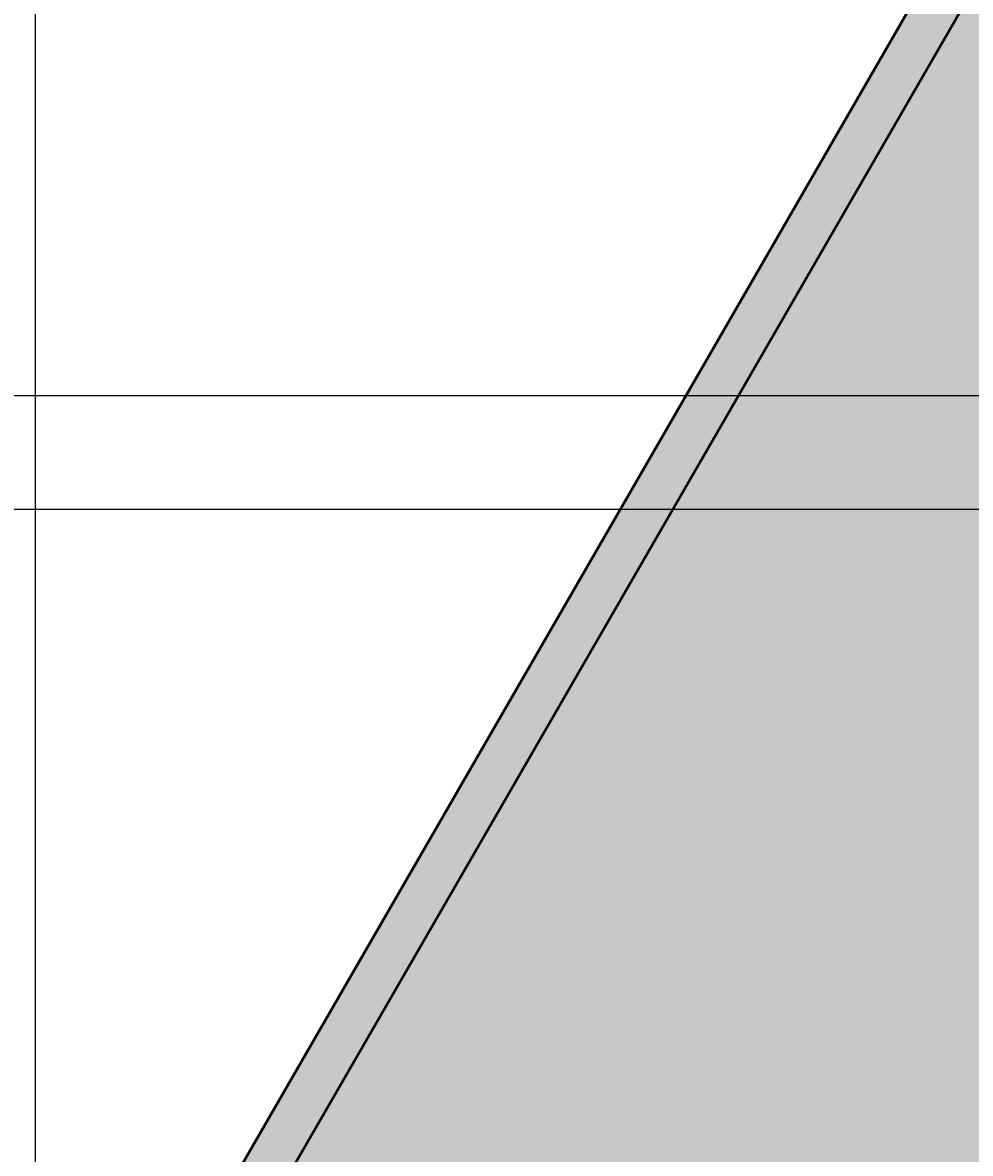
# Model space of a CAD drawing. Units: inches. Extents: x -12 to 334, y -10 to 186.
# Tile 57 of 77: x 106 to 127, y 111 to 136. Entities that reach past the tile are written whole.
import ezdxf
from ezdxf import colors
from ezdxf.entities.mleader import LeaderData, LeaderLine
from ezdxf.math import Vec2, Vec3

# ---------------------------------------------------------------- set-up
doc = ezdxf.new("R2010")
doc.units = ezdxf.units.IN
doc.header["$MEASUREMENT"] = 0
for name, color, linetype, lineweight in [('M-ANNO-TEXT', 3, 'Continuous', 25), ('M-DIMS', 2, 'Continuous', 18), ('M-EQPM', 7, 'Continuous', 50), ('M-EQPM-PATT', 8, 'Continuous', 18)]:
    doc.layers.add(name, color=color, linetype=linetype, lineweight=lineweight)
doc.styles.get("Standard").update_dxf_attribs({"font": 'arial.ttf'})
doc.dimstyles.get("Standard").update_dxf_attribs({"dimtxt": 0.18, "dimasz": 0.18, "dimexe": 0.18, "dimexo": 0.0625, "dimgap": 0.09, "dimtad": 0, "dimtih": 1, "dimtoh": 1, "dimdec": 4, "dimzin": 0, "dimdsep": 46, "dimtxsty": 'Standard', "dimcen": 0.09, "dimadec": 0, "dimazin": 0, "dimtfac": 1, "dimtdec": 4, "dimtofl": 0, "dimtmove": 0, "dimatfit": 3, "dimfxl": 1, "dimtolj": 1, "dimtzin": 0, "dimarcsym": 0})

# ---------------------------------------------------------------- blocks, each defined once
blk = doc.blocks.new('*D5')
at = {"layer": 'Defpoints', "color": 0, "transparency": 16777216}
for p in [(58.1, 127.708), (58.1, 125.208), (295.976, 125.208)]:
    blk.add_point(p, dxfattribs=at)
at = {"layer": 'M-DIMS', "color": 0, "lineweight": -2, "transparency": 16777216}
for p, q in [((58.163, 127.708), (296.156, 127.708)), ((295.976, 127.528), (295.976, 126.64)), ((295.976, 125.388), (295.976, 126.276)), ((58.163, 125.208), (296.156, 125.208))]:
    blk.add_line(p, q, dxfattribs=at)
at = {"layer": 'M-DIMS', "color": 0, "transparency": 16777216}
for points in [[(295.946, 127.528), (296.006, 127.528), (295.976, 127.708)], [(295.946, 125.388), (296.006, 125.388), (295.976, 125.208)]]:
    blk.add_solid(points, dxfattribs=at)
at = {"layer": 'M-DIMS', "color": 0, "transparency": 16777216, "insert": (295.976, 126.458), "char_height": 0.18, "attachment_point": 5}
blk.add_mtext('\\A1;2.5', dxfattribs=at)
blk = doc.blocks.new('*D15')
at = {"layer": 'Defpoints', "color": 0, "transparency": 16777216}
for p in [(106.177, 169.385), (86.888, 109.058), (106.177, 102.896)]:
    blk.add_point(p, dxfattribs=at)
at = {"layer": 'M-DIMS', "color": 0, "lineweight": -2, "transparency": 16777216}
for p, q in [((86.888, 109.121), (86.888, 169.565)), ((87.068, 169.385), (96.147, 169.385)), ((105.997, 169.385), (96.918, 169.385)), ((106.177, 102.958), (106.177, 169.565))]:
    blk.add_line(p, q, dxfattribs=at)
at = {"layer": 'M-DIMS', "color": 0, "transparency": 16777216}
for points in [[(87.068, 169.415), (87.068, 169.355), (86.888, 169.385)], [(105.997, 169.415), (105.997, 169.355), (106.177, 169.385)]]:
    blk.add_solid(points, dxfattribs=at)
at = {"layer": 'M-DIMS', "color": 0, "transparency": 16777216, "insert": (96.532, 169.385), "char_height": 0.18, "attachment_point": 5}
blk.add_mtext('\\A1;19.29', dxfattribs=at)
blk = doc.blocks.new('*D16')
at = {"layer": 'Defpoints', "color": 0, "transparency": 16777216}
for p in [(126.379, 169.385), (126.379, 137.887), (106.177, 102.896)]:
    blk.add_point(p, dxfattribs=at)
at = {"layer": 'M-DIMS', "color": 0, "lineweight": -2, "transparency": 16777216}
for p, q in [((106.177, 102.958), (106.177, 169.565)), ((106.357, 169.385), (115.814, 169.385)), ((126.199, 169.385), (116.742, 169.385)), ((126.379, 137.95), (126.379, 169.565))]:
    blk.add_line(p, q, dxfattribs=at)
at = {"layer": 'M-DIMS', "color": 0, "transparency": 16777216}
for points in [[(106.357, 169.415), (106.357, 169.355), (106.177, 169.385)], [(126.199, 169.415), (126.199, 169.355), (126.379, 169.385)]]:
    blk.add_solid(points, dxfattribs=at)
at = {"layer": 'M-DIMS', "color": 0, "transparency": 16777216, "insert": (116.278, 169.385), "char_height": 0.18, "attachment_point": 5}
blk.add_mtext('\\A1;20.202', dxfattribs=at)

msp = doc.modelspace()

# ---------------------------------------------------------------- hatches: boundary and pattern name
at = {"layer": 'M-EQPM-PATT', "transparency": 33554556}
h = msp.add_hatch(color=256, dxfattribs=at)
h.set_gradient(color1=(248, 206, 179), color2=(248, 206, 179), tint=1)
h.paths.add_polyline_path([(179.7818, 136.8871), (126.9567, 136.8871), (106.1771, 100.8958), (171.5458, 100.8958)])
h.paths.add_polyline_path([(268.3808, 136.9435), (214.0166, 136.9435), (214.0166, 154.8345), (196.3421, 154.8345), (196.3421, 136.8871), (179.7818, 136.8871), (171.5458, 100.8958), (231.7758, 100.8958, -0.4142136), (251.9801, 80.6915), (279.7263, 80.6915, 0.1631825)])
at = {"layer": 'M-EQPM-PATT'}
h = msp.add_hatch(color=256, dxfattribs=at)
h.set_gradient(color1=(99, 100, 102), color2=(99, 100, 102), tint=1)
h.paths.add_polyline_path([(126.9567, 136.8871), (179.7818, 136.8871), (180.0106, 137.8871), (126.3793, 137.8871), (106.1771, 102.8958), (86.8879, 102.8958), (86.8879, 109.0583), (84.7229, 109.0583), (84.7229, 100.8958), (106.1771, 100.8958)])
h.paths.add_polyline_path([(196.3421, 152.8345), (195.3421, 152.8345), (195.3421, 137.8871), (180.0106, 137.8871), (179.7818, 136.8871), (196.3421, 136.8871)])
h.paths.add_polyline_path([(215.0166, 152.8345), (214.0166, 152.8345), (214.0166, 136.9435), (268.3808, 136.9435, -0.2673785), (268.3808, 46.8541), (249.3759, 46.8541), (249.8485, 45.8541), (269.3808, 45.8541, 0.2615891), (269.3808, 137.9435), (215.0166, 137.9435)])

# ---------------------------------------------------------------- linework, layer by layer
at = {"layer": 'M-EQPM'}
for points in [[(106.1771, 100.8958), (126.9567, 136.8871), (196.3421, 136.8871), (196.3421, 154.8345)], [(106.1771, 102.8958), (126.3793, 137.8871), (195.3421, 137.8871), (195.3421, 152.8345)]]:
    msp.add_lwpolyline(points, dxfattribs=at)

# ---------------------------------------------------------------- dimensions: what is measured, and where the dimension line sits
at = {"layer": 'M-DIMS'}
for base, p1, p2, override, picture, middle in [((106.1771, 169.3845), (86.8879, 109.0583), (106.1771, 102.8958), {"dimdec": 2, "dimlfac": 1, "dimrnd": 0, "dimzin": 0, "dimdsep": 46, "dimlunit": 2}, '*D15', (96.5325, 169.3845)), ((126.3793, 169.3845), (106.1771, 102.8958), (126.3793, 137.8871), {"dimdec": 3, "dimlfac": 1, "dimrnd": 0, "dimzin": 0, "dimdsep": 46, "dimlunit": 2}, '*D16', (116.2782, 169.3845))]:
    dim = msp.add_linear_dim(base=base, p1=p1, p2=p2, dimstyle='Standard', override=override, dxfattribs=at)
    dim.commit()
    dim.dimension.update_dxf_attribs({"geometry": picture, "text_midpoint": middle})
dim = msp.add_linear_dim(base=(295.9756, 125.2078), p1=(58.1002, 127.7078), p2=(58.1002, 125.2078), angle=90, dimstyle='Standard', override={"dimdec": 1, "dimlfac": 1, "dimrnd": 0, "dimzin": 0, "dimdsep": 46, "dimlunit": 2}, dxfattribs=at)
dim.commit()
dim.dimension.update_dxf_attribs({"geometry": '*D5', "text_midpoint": (295.9756, 126.4578)})

# ---------------------------------------------------------------- leaders
at = {"layer": 'M-ANNO-TEXT'}
ml = msp.add_multileader_mtext('Standard', dxfattribs=at)
ml.set_content('Tube plate', color=256)
ml.set_leader_properties()
ml.build(insert=Vec2(0, 0))
ml.multileader.update_dxf_attribs({"dogleg_length": 0.36, "arrow_head_size": 0.7})
ctx = ml.context
ctx.base_point, ctx.arrow_head_size, ctx.landing_gap_size, ctx.plane_origin = Vec3(95.9742, 157.4218), 0.7, 0.09, Vec3(31.4743, 171.7024)
notes = []
notes.append((ctx, [(0, (1, 1, 0), (78.5354, 157.4218), (1, 0), 17.4388, [(0, [(75.9244, 109.0583)], 0, [])])]))
ctx.mtext.insert, ctx.mtext.flow_direction = Vec3(96.0642, 159.9771), 5
for ctx, leaders in notes:
    for number, flags, end, landing, length, lines in leaders:
        leader = LeaderData()
        leader.index, (leader.has_last_leader_line, leader.has_dogleg_vector, leader.attachment_direction) = number, flags
        leader.last_leader_point, leader.dogleg_vector, leader.dogleg_length = Vec3(end), Vec3(landing), length
        for number, points, colour, breaks in lines:
            line = LeaderLine()
            line.index, line.vertices, line.color, line.breaks = number, Vec3.list(points), colors.encode_raw_color(colour), breaks
            leader.lines.append(line)
        ctx.leaders.append(leader)

doc.saveas('drawing.dxf')
